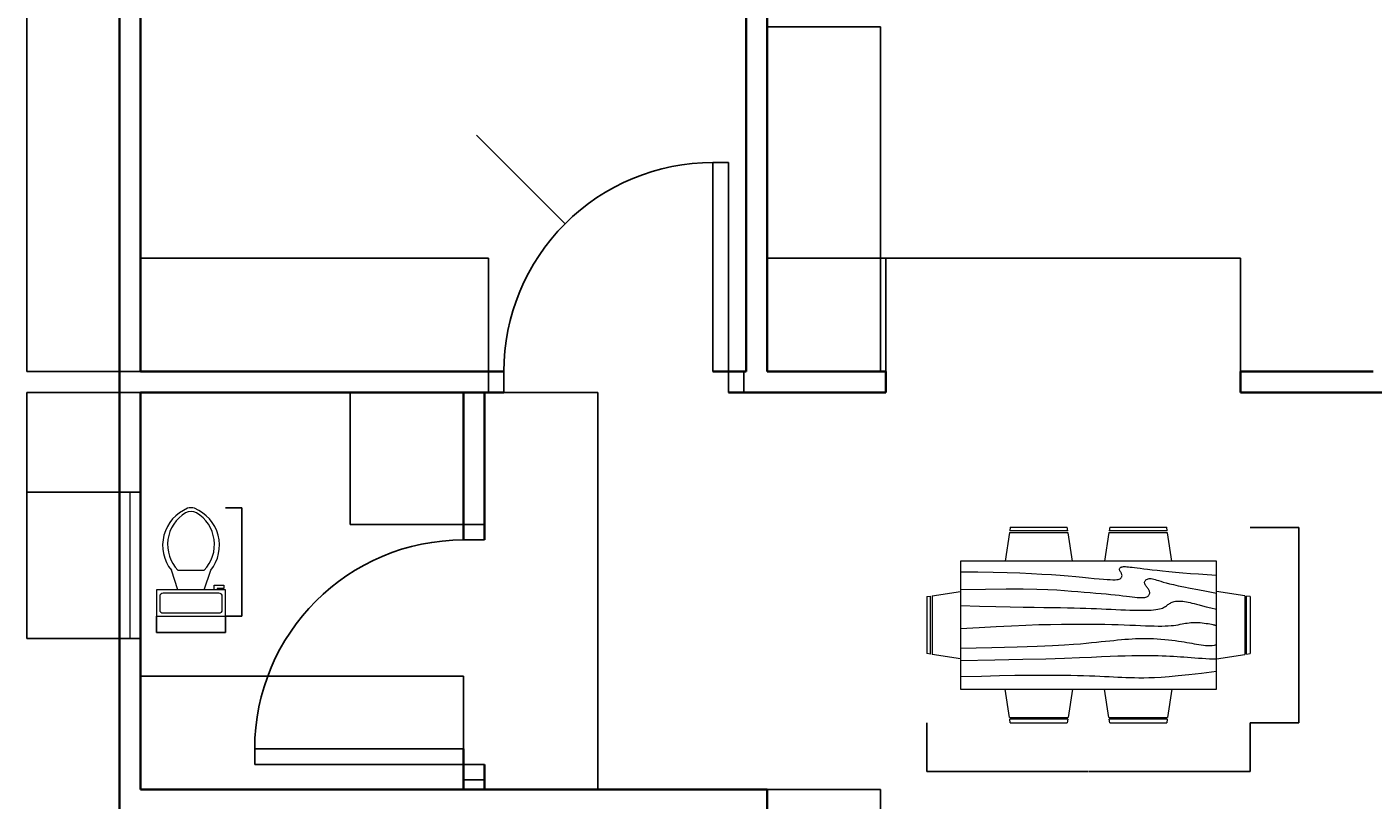
# Model space of a CAD drawing. Units: millimetres. Extents: x 1426 to 11512, y -8522 to 2664.
# Tile 2 of 4: x 1426 to 7869, y -3929 to -230. Entities that reach past the tile are written whole.
import ezdxf

# ---------------------------------------------------------------- set-up
doc = ezdxf.new("R2010")
doc.units = ezdxf.units.MM
for name, color, linetype, lineweight in [('A-ANNO-DIMS', 2, 'Continuous', 18), ('A-DOOR', 3, 'Continuous', 25), ('A-FLOR-FIXT', 9, 'Continuous', 20), ('A-FURN', 8, 'Continuous', 18), ('A-GLAZ', 4, 'Continuous', 18), ('A-WALL', 7, 'Continuous', 35)]:
    doc.layers.add(name, color=color, linetype=linetype, lineweight=lineweight)
doc.styles.get("Standard").update_dxf_attribs({"font": 'arial.ttf'})
doc.dimstyles.get("Standard").update_dxf_attribs({"dimtxt": 0.18, "dimasz": 0.18, "dimexe": 0.18, "dimexo": 0.0625, "dimgap": 0.09, "dimtad": 0, "dimtih": 1, "dimtoh": 1, "dimdec": 4, "dimzin": 0, "dimdsep": 46, "dimtxsty": 'Standard', "dimcen": 0.09, "dimadec": 0, "dimazin": 0, "dimtfac": 1, "dimtdec": 4, "dimtofl": 0, "dimtmove": 0, "dimatfit": 3, "dimfxl": 1, "dimtolj": 1, "dimtzin": 0, "dimarcsym": 0})

# ---------------------------------------------------------------- blocks, each defined once
blk = doc.blocks.new('Dining Set - 36 x 72 in.')
for p, q in [((-22, 27.5), (-22.1562, 26.50042)), ((-22, 27.5), (-6, 27.5)), ((-5.8437, 26.49966), (-6, 27.5)), ((6, 27.5), (5.8438, 26.50042)), ((6, 27.5), (22, 27.5)), ((22.1563, 26.49966), (22, 27.5)), ((-22.2343, 26.00059), (-23.4847, 17.99762)), ((-22.2304, 26), (-5.7608, 26)), ((-5.8416, 26.5), (-22.1534, 26.5)), ((-4.5152, 17.99762), (-5.7655, 25.99926)), ((5.7657, 26.00059), (4.5153, 17.99762)), ((5.7696, 26), (22.2392, 26)), ((22.1584, 26.5), (5.8466, 26.5)), ((23.4848, 17.99762), (22.2345, 25.99926)), ((36, 18), (-36, 18)), ((-36, 18), (-36, -18)), ((36, -18), (36, 18)), ((-45.5, 8), (-44.5004, 8.15617)), ((-45.5, 8), (-45.5, -8)), ((-44.5, -8.15843), (-44.5, 8.15338)), ((-44.0006, 8.23428), (-35.9976, 9.48474)), ((-44, 8.23041), (-44, -8.23915)), ((44.0006, 8.23428), (35.9976, 9.48474)), ((44, 8.23041), (44, -8.23915)), ((44.5, -8.15843), (44.5, 8.15338)), ((45.5, 8), (44.5005, 8.15617)), ((45.5, 8), (45.5, -8)), ((-44.4997, -8.15631), (-45.5, -8)), ((-35.9976, -9.48476), (-43.9993, -8.2345)), ((35.9976, -9.48476), (43.9993, -8.2345)), ((44.4997, -8.15631), (45.5, -8)), ((-36, -18), (36, -18)), ((-22.2343, -26.0006), (-23.4847, -17.99762)), ((-4.5152, -17.99762), (-5.7655, -25.99928)), ((5.7657, -26.0006), (4.5153, -17.99762)), ((23.4848, -17.99762), (22.2345, -25.99928)), ((-22.2304, -26), (-5.7608, -26)), ((-22, -27.5), (-22.1562, -26.50044)), ((-5.8416, -26.5), (-22.1534, -26.5)), ((-5.8437, -26.49967), (-6, -27.5)), ((5.7696, -26), (22.2392, -26)), ((6, -27.5), (5.8438, -26.50044)), ((22.1584, -26.5), (5.8466, -26.5)), ((22.1563, -26.49967), (22, -27.5)), ((-22, -27.5), (-6, -27.5)), ((6, -27.5), (22, -27.5))]:
    blk.add_line(p, q)
for points in [[(-36, 15), (-31.1772, 14.97754), (-26.8079, 14.91406), (-22.8538, 14.81543), (-19.276, 14.6875), (-16.0362, 14.53613), (-13.0957, 14.36718), (-10.4159, 14.18652), (-7.9583, 14), (-5.6904, 13.81315), (-3.6035, 13.63021), (-1.6954, 13.45508), (0.0365, 13.29166), (1.5945, 13.14388), (2.9811, 13.01562), (4.1988, 12.9108), (5.25, 12.83333), (6.1393, 12.78613), (6.8802, 12.76823), (7.4883, 12.77767), (7.9792, 12.8125), (8.3685, 12.87077), (8.6719, 12.95052), (8.9049, 13.0498), (9.0833, 13.16666), (9.2205, 13.29899), (9.3216, 13.44401), (9.3895, 13.59879), (9.4271, 13.76041), (9.4373, 13.92594), (9.4232, 14.09245), (9.3875, 14.257), (9.3333, 14.41666), (9.2638, 14.56917), (9.1836, 14.71484), (9.0975, 14.85465), (9.0104, 14.98958), (8.9272, 15.1206), (8.8529, 15.2487), (8.7922, 15.37483), (8.75, 15.5), (8.7305, 15.62467), (8.7344, 15.74739), (8.7617, 15.86621), (8.8125, 15.97916), (8.8867, 16.08431), (8.9844, 16.17968), (9.1055, 16.26334), (9.25, 16.33333), (9.4189, 16.38802), (9.6172, 16.42708), (9.8506, 16.45052), (10.125, 16.45833), (10.4463, 16.45052), (10.8203, 16.42708), (11.2529, 16.38802), (11.75, 16.33333), (12.3184, 16.26318), (12.9694, 16.17838), (13.7151, 16.07991), (14.5677, 15.96875), (15.5395, 15.84586), (16.6426, 15.71224), (17.8893, 15.56884), (19.2917, 15.41666), (20.859, 15.25667), (22.5879, 15.08984), (24.4721, 14.91715), (26.5052, 14.73958), (28.6809, 14.5581), (30.9929, 14.3737), (33.4347, 14.18733), (36, 14)], [(-36, 10), (-28.9766, 10.14274), (-23.1725, 10.20442), (-18.4241, 10.19775), (-14.5677, 10.13541), (-11.4399, 10.03011), (-8.877, 9.89453), (-6.7154, 9.74137), (-4.7917, 9.58333), (-2.9698, 9.43082), (-1.2246, 9.28515), (0.4415, 9.14534), (2.026, 9.01041), (3.5266, 8.87939), (4.9408, 8.7513), (6.266, 8.62516), (7.5, 8.5), (8.6411, 8.37549), (9.6914, 8.2539), (10.6538, 8.13818), (11.5312, 8.03125), (12.3267, 7.93603), (13.043, 7.85547), (13.6831, 7.79248), (14.25, 7.75), (14.7471, 7.7303), (15.1797, 7.73307), (15.5537, 7.75732), (15.875, 7.80208), (16.1494, 7.86637), (16.3828, 7.94922), (16.5811, 8.04964), (16.75, 8.16666), (16.8944, 8.29915), (17.0143, 8.44531), (17.1089, 8.60319), (17.1771, 8.77083), (17.218, 8.94629), (17.2305, 9.1276), (17.2137, 9.31282), (17.1667, 9.5), (17.0895, 9.6875), (16.987, 9.875), (16.8649, 10.0625), (16.7292, 10.25), (16.5856, 10.4375), (16.4401, 10.625), (16.2985, 10.8125), (16.1667, 11), (16.05, 11.18733), (15.9518, 11.3737), (15.8752, 11.5581), (15.8229, 11.73958), (15.798, 11.91715), (15.8034, 12.08984), (15.842, 12.25667), (15.9167, 12.41666), (16.0295, 12.56836), (16.1784, 12.70833), (16.3605, 12.83268), (16.5729, 12.9375), (16.8127, 13.01888), (17.0768, 13.07291), (17.3625, 13.0957), (17.6667, 13.08333), (17.9894, 13.03312), (18.3418, 12.94726), (18.7382, 12.82918), (19.1927, 12.68229), (19.7195, 12.51001), (20.3327, 12.31575), (21.0465, 12.10294), (21.875, 11.875), (22.8357, 11.63354), (23.959, 11.37304), (25.2786, 11.08618), (26.8282, 10.76562), (28.6414, 10.40405), (30.752, 9.99414), (33.1936, 9.52856), (36, 9)], [(-36, 5.5), (-30.7157, 5.3348), (-26.069, 5.20963), (-21.9946, 5.11767), (-18.4271, 5.05208), (-15.3009, 5.00602), (-12.5508, 4.97265), (-10.1112, 4.94515), (-7.9167, 4.91666), (-5.909, 4.88167), (-4.0586, 4.83984), (-2.3429, 4.79215), (-0.7396, 4.73958), (0.7739, 4.6831), (2.22, 4.6237), (3.6213, 4.56233), (5, 4.5), (6.373, 4.43782), (7.7344, 4.3776), (9.0723, 4.32129), (10.375, 4.27083), (11.6309, 4.22819), (12.8281, 4.19531), (13.9551, 4.17415), (15, 4.16666), (15.954, 4.17448), (16.819, 4.19791), (17.6001, 4.23698), (18.3021, 4.29166), (18.9299, 4.36198), (19.4883, 4.44791), (19.9823, 4.54948), (20.4167, 4.66666), (20.7969, 4.79899), (21.1302, 4.94401), (21.4245, 5.09879), (21.6875, 5.26041), (21.9271, 5.42594), (22.1511, 5.59245), (22.3672, 5.757), (22.5834, 5.91666), (22.8065, 6.06868), (23.0404, 6.21093), (23.2879, 6.34147), (23.5521, 6.45833), (23.8358, 6.55957), (24.142, 6.64323), (24.4735, 6.70735), (24.8334, 6.75), (25.2235, 6.76969), (25.642, 6.76692), (26.0858, 6.74267), (26.5521, 6.69791), (27.0379, 6.63362), (27.5404, 6.55078), (28.0565, 6.45036), (28.5834, 6.33333), (29.1242, 6.19987), (29.7071, 6.04687), (30.3661, 5.87044), (31.1354, 5.66666), (32.0493, 5.43164), (33.142, 5.16146), (34.4475, 4.85221), (36, 4.5)], [(-36, -1), (-30.7915, -0.6591), (-26.0195, -0.38216), (-21.6519, -0.16284), (-17.6563, 0.00521), (-14.0005, 0.12833), (-10.6523, 0.21289), (-7.5796, 0.26522), (-4.75, 0.29166), (-2.134, 0.29793), (0.2878, 0.28711), (2.5317, 0.26163), (4.6146, 0.22396), (6.5529, 0.17651), (8.3633, 0.12174), (10.0623, 0.06209), (11.6667, 0), (13.1899, -0.06201), (14.6341, -0.1211), (15.9982, -0.17432), (17.2813, -0.21875), (18.4823, -0.25147), (19.6003, -0.26953), (20.6343, -0.27002), (21.5834, -0.25), (22.4481, -0.20768), (23.2357, -0.14584), (23.9549, -0.06836), (24.6146, 0.02083), (25.2235, 0.11784), (25.7904, 0.21875), (26.3241, 0.31966), (26.8334, 0.41666), (27.3265, 0.50618), (27.8099, 0.58593), (28.2894, 0.65397), (28.7709, 0.70833), (29.2601, 0.74707), (29.763, 0.76823), (30.2855, 0.76985), (30.8334, 0.75), (31.4088, 0.70784), (31.9994, 0.64713), (32.589, 0.57275), (33.1615, 0.48958), (33.7008, 0.4025), (34.1908, 0.3164), (34.6153, 0.23616), (34.9584, 0.16666), (35.2099, 0.11165), (35.3848, 0.07031), (35.504, 0.04069), (35.5886, 0.02083), (35.6594, 0.00879), (35.7377, 0.0026), (35.8442, 0.00032), (36, 0)], [(-36, -6.5), (-27.1843, -6.31267), (-20.084, -6.1263), (-14.469, -5.9419), (-10.1094, -5.76042), (-6.7752, -5.58285), (-4.2363, -5.41016), (-2.2629, -5.24333), (-0.625, -5.08334), (0.8708, -4.93099), (2.2715, -4.78646), (3.5872, -4.64974), (4.8281, -4.52084), (6.0046, -4.39974), (7.127, -4.28646), (8.2053, -4.18099), (9.25, -4.08334), (10.2705, -3.99382), (11.2734, -3.91407), (12.2647, -3.84603), (13.25, -3.79167), (14.2354, -3.75293), (15.2266, -3.73177), (16.2295, -3.73015), (17.25, -3.75), (18.2912, -3.79248), (19.3451, -3.85547), (20.4009, -3.93604), (21.4479, -4.03125), (22.4754, -4.13819), (23.4727, -4.25391), (24.4289, -4.37549), (25.3334, -4.5), (26.1785, -4.62492), (26.9694, -4.74935), (27.7145, -4.87281), (28.4219, -4.99479), (29.1, -5.11483), (29.7572, -5.23242), (30.4016, -5.34709), (31.0417, -5.45834), (31.6837, -5.56437), (32.3262, -5.65821), (32.9658, -5.73153), (33.599, -5.77604), (34.2224, -5.78345), (34.8327, -5.74545), (35.4264, -5.65373), (36, -5.5)], [(-36, -10), (-26.4022, -9.81299), (-18.4675, -9.62891), (-11.9839, -9.45069), (-6.7396, -9.28125), (-2.5226, -9.12354), (0.8789, -8.98047), (3.6769, -8.85498), (6.0833, -8.75), (8.2767, -8.66765), (10.3021, -8.60677), (12.1712, -8.56543), (13.8958, -8.54167), (15.4876, -8.53353), (16.9583, -8.53907), (18.3197, -8.55632), (19.5834, -8.58334), (20.7616, -8.61841), (21.8685, -8.66081), (22.9188, -8.71004), (23.9271, -8.76563), (24.9081, -8.82707), (25.8763, -8.89388), (26.8465, -8.96558), (27.8334, -9.04167), (28.8474, -9.12118), (29.8828, -9.20117), (30.93, -9.27824), (31.9792, -9.34896), (33.0205, -9.40991), (34.0443, -9.45768), (35.0407, -9.48885), (36, -9.5)], [(-36, -14.5), (-30.0881, -14.33513), (-25.0332, -14.21224), (-20.7312, -14.12647), (-17.0781, -14.07292), (-13.97, -14.04671), (-11.3027, -14.04297), (-8.9724, -14.05681), (-6.875, -14.08334), (-4.9224, -14.11833), (-3.0905, -14.16016), (-1.3709, -14.20785), (0.2448, -14.26042), (1.7647, -14.3169), (3.1973, -14.3763), (4.5507, -14.43767), (5.8333, -14.5), (7.0554, -14.5621), (8.235, -14.62175), (9.3922, -14.67652), (10.5469, -14.72396), (11.7192, -14.76164), (12.929, -14.78711), (14.1965, -14.79794), (15.5417, -14.79167), (16.9933, -14.76424), (18.6152, -14.70508), (20.4804, -14.60197), (22.6615, -14.44271), (25.2312, -14.21509), (28.2624, -13.9069), (31.8277, -13.50594), (36, -13)]]:
    blk.add_lwpolyline(points)
blk = doc.blocks.new('Toilet - top')
for p, q in [((9.5, -6), (9.5, -2)), ((-8, -8.5), (-8, -8)), ((-7, -8), (-7, -9.5)), ((-4, -8), (-6, -14)), ((4, -8), (6, -14)), ((-10, -8.5), (-8, -8.5)), ((-10, -9.5), (-10, -8.5)), ((-7, -9.5), (-10, -9.5)), ((4, -14), (-4, -14))]:
    blk.add_line(p, q)
blk.add_lwpolyline([(10.5, -8), (10.5, 0), (-10.5, 0), (-10.5, -8)], close=True)
for points in [[(-9.5, -2), (-9.5, -6)], [(8.5, -1), (-8.5, -1)], [(-8.5, -7), (8.5, -7)]]:
    blk.add_lwpolyline(points)
for centre, radius, start, end in [((-8.62, -1.88), 0.884, 81.8699, 188.1301), ((8.62, -1.88), 0.884, 351.8699, 98.1301), ((-8.62, -6.12), 0.884, 171.8699, 278.1301), ((8.62, -6.12), 0.884, 261.8699, 8.1301), ((3.52, -21.58), 12.17, 141.4691, 247.9714), ((4.2, -21.82), 11.33, 136.3677, 238.9468), ((-3.52, -21.58), 12.17, 292.0284, 38.5307), ((-4.2, -21.82), 11.33, 301.053, 43.6321), ((0, -27.88), 4, 245.7318, 294.2682), ((0, -29), 4, 254.8605, 285.1395)]:
    blk.add_arc(centre, radius, start, end)
blk = doc.blocks.new('DOOR-SINGLE-1000')
for p, q in [((0, 1000), (0, 1100)), ((0, 1100), (74.2, 1100)), ((74.2, 1100), (74.2, 1000)), ((1148.4, 1000), (1148.4, 1100)), ((1148.4, 1100), (1222.6, 1100)), ((1222.6, 1100), (1222.6, 1000)), ((74.2, 1000), (0, 1000)), ((74.2, 1000), (148.4, 1000)), ((74.2, 0), (74.2, 1000)), ((148.4, 1000), (148.4, 0)), ((1222.6, 1000), (1148.4, 1000)), ((148.4, 0), (74.2, 0))]:
    blk.add_line(p, q)
blk.add_arc((148.4, 1000), 1000, 270, 0)
blk = doc.blocks.new('DOOR-LEAF-1000')
for p, q in [((1000, 74.2), (0, 74.2)), ((0, 74.2), (0, 0)), ((1000, 0), (1000, 74.2)), ((0, 0), (1000, 0))]:
    blk.add_line(p, q)
blk.add_arc((1000, 74.2), 1000, 90, 180)
blk = doc.blocks.new('*D32')
at = {"layer": 'A-ANNO-DIMS', "color": 0, "lineweight": -2, "transparency": 16777216}
for p, q in [((5733, -3559.8), (5733, -3792)), ((7280.7, -3559.8), (7280.7, -3792)), ((5733.1, -3791.8), (6505.7, -3791.8)), ((7280.5, -3791.8), (6507.9, -3791.8))]:
    blk.add_line(p, q, dxfattribs=at)
at = {"layer": 'A-ANNO-DIMS', "color": 0, "transparency": 16777216}
for points in [[(5733.1, -3791.8), (5733.1, -3791.9), (5733, -3791.8)], [(7280.5, -3791.8), (7280.5, -3791.9), (7280.7, -3791.8)]]:
    blk.add_solid(points, dxfattribs=at)
at = {"layer": 'Defpoints', "color": 0, "transparency": 16777216}
for p in [(5733, -3559.7), (7280.7, -3559.7), (7280.7, -3791.8)]:
    blk.add_point(p, dxfattribs=at)
at = {"layer": 'A-ANNO-DIMS', "color": 0, "transparency": 16777216, "insert": (6506.8, -3791.8), "char_height": 0.18, "attachment_point": 5}
blk.add_mtext('\\A1;DINING SET 1548', dxfattribs=at)
blk = doc.blocks.new('*D33')
at = {"layer": 'A-ANNO-DIMS', "color": 0, "lineweight": -2, "transparency": 16777216}
for p, q in [((7280.7, -2624.3), (7513, -2624.3)), ((7512.8, -2624.4), (7512.8, -3091.8)), ((7512.8, -3559.5), (7512.8, -3092.2)), ((7280.7, -3559.7), (7513, -3559.7))]:
    blk.add_line(p, q, dxfattribs=at)
at = {"layer": 'A-ANNO-DIMS', "color": 0, "transparency": 16777216}
for points in [[(7512.8, -2624.4), (7512.8, -2624.4), (7512.8, -2624.3)], [(7512.8, -3559.5), (7512.8, -3559.5), (7512.8, -3559.7)]]:
    blk.add_solid(points, dxfattribs=at)
at = {"layer": 'Defpoints', "color": 0, "transparency": 16777216}
for p in [(7280.7, -2624.3), (7512.8, -2624.3), (7280.7, -3559.7)]:
    blk.add_point(p, dxfattribs=at)
at = {"layer": 'A-ANNO-DIMS', "color": 0, "transparency": 16777216, "insert": (7512.8, -3092), "char_height": 0.18, "attachment_point": 5}
blk.add_mtext('\\A1;935', dxfattribs=at)
blk = doc.blocks.new('*D34')
at = {"layer": 'A-ANNO-DIMS', "color": 0, "lineweight": -2, "transparency": 16777216}
for p, q in [((2376.6, -2530.4), (2454.6, -2530.4)), ((2454.4, -2530.6), (2454.4, -2789.9)), ((2454.4, -3049.6), (2454.4, -2790.3)), ((2376.6, -3049.8), (2454.6, -3049.8))]:
    blk.add_line(p, q, dxfattribs=at)
at = {"layer": 'A-ANNO-DIMS', "color": 0, "transparency": 16777216}
for points in [[(2454.4, -2530.6), (2454.5, -2530.6), (2454.4, -2530.4)], [(2454.4, -3049.6), (2454.5, -3049.6), (2454.4, -3049.8)]]:
    blk.add_solid(points, dxfattribs=at)
at = {"layer": 'Defpoints', "color": 0, "transparency": 16777216}
for p in [(2376.5, -2530.4), (2376.5, -3049.8), (2454.4, -3049.8)]:
    blk.add_point(p, dxfattribs=at)
at = {"layer": 'A-ANNO-DIMS', "color": 0, "transparency": 16777216, "insert": (2454.4, -2790.1), "char_height": 0.18, "attachment_point": 5}
blk.add_mtext('\\A1;WC 519', dxfattribs=at)
blk = doc.blocks.new('*D35')
at = {"layer": 'A-ANNO-DIMS', "color": 0, "lineweight": -2, "transparency": 16777216}
for p, q in [((2046.5, -3049.8), (2046.5, -3127.8)), ((2376.5, -3049.8), (2376.5, -3127.8)), ((2046.7, -3127.7), (2211.3, -3127.7)), ((2376.4, -3127.7), (2211.8, -3127.7))]:
    blk.add_line(p, q, dxfattribs=at)
at = {"layer": 'A-ANNO-DIMS', "color": 0, "transparency": 16777216}
for points in [[(2046.7, -3127.6), (2046.7, -3127.7), (2046.5, -3127.7)], [(2376.4, -3127.6), (2376.4, -3127.7), (2376.5, -3127.7)]]:
    blk.add_solid(points, dxfattribs=at)
at = {"layer": 'Defpoints', "color": 0, "transparency": 16777216}
for p in [(2046.5, -3049.8), (2376.5, -3049.8), (2046.5, -3127.7)]:
    blk.add_point(p, dxfattribs=at)
at = {"layer": 'A-ANNO-DIMS', "color": 0, "transparency": 16777216, "insert": (2211.5, -3127.7), "char_height": 0.18, "attachment_point": 5}
blk.add_mtext('\\A1;330', dxfattribs=at)
blk = doc.blocks.new('*D43')
at = {"layer": 'A-ANNO-DIMS', "color": 0, "lineweight": -2, "transparency": 16777216}
for p, q in [((1968.8, 2020.9), (1426.2, 2020.9)), ((1426.4, 2020.8), (1426.4, 71.1)), ((1426.4, -1878.9), (1426.4, 70.8)), ((1968.8, -1879.1), (1426.2, -1879.1))]:
    blk.add_line(p, q, dxfattribs=at)
at = {"layer": 'A-ANNO-DIMS', "color": 0, "transparency": 16777216}
for points in [[(1426.3, 2020.8), (1426.4, 2020.8), (1426.4, 2020.9)], [(1426.3, -1878.9), (1426.4, -1878.9), (1426.4, -1879.1)]]:
    blk.add_solid(points, dxfattribs=at)
at = {"layer": 'Defpoints', "color": 0, "transparency": 16777216}
for p in [(1426.4, 2020.9), (1968.9, 2020.9), (1968.9, -1879.1)]:
    blk.add_point(p, dxfattribs=at)
at = {"layer": 'A-ANNO-DIMS', "color": 0, "transparency": 16777216, "insert": (1426.4, 70.9), "char_height": 0.18, "attachment_point": 5}
blk.add_mtext('\\A1;3900', dxfattribs=at)
blk = doc.blocks.new('*D44')
at = {"layer": 'A-ANNO-DIMS', "color": 0, "lineweight": -2, "transparency": 16777216}
for p, q in [((3616.2, -1979.1), (4158.8, -1979.1)), ((4158.6, -1979.2), (4158.6, -2928.9)), ((4158.6, -3878.9), (4158.6, -2929.2)), ((3616.2, -3879.1), (4158.8, -3879.1))]:
    blk.add_line(p, q, dxfattribs=at)
at = {"layer": 'A-ANNO-DIMS', "color": 0, "transparency": 16777216}
for points in [[(4158.6, -1979.2), (4158.7, -1979.2), (4158.6, -1979.1)], [(4158.6, -3878.9), (4158.7, -3878.9), (4158.6, -3879.1)]]:
    blk.add_solid(points, dxfattribs=at)
at = {"layer": 'Defpoints', "color": 0, "transparency": 16777216}
for p in [(3616.1, -1979.1), (3616.1, -3879.1), (4158.6, -3879.1)]:
    blk.add_point(p, dxfattribs=at)
at = {"layer": 'A-ANNO-DIMS', "color": 0, "transparency": 16777216, "insert": (4158.6, -2929.1), "char_height": 0.18, "attachment_point": 5}
blk.add_mtext('\\A1;1900', dxfattribs=at)
blk = doc.blocks.new('*D46')
at = {"layer": 'A-ANNO-DIMS', "color": 0, "lineweight": -2, "transparency": 16777216}
for p, q in [((1968.9, -3879), (1968.9, -3336.4)), ((1969.1, -3336.6), (2742, -3336.6)), ((3515.9, -3336.6), (2743, -3336.6)), ((3516.1, -3879), (3516.1, -3336.4))]:
    blk.add_line(p, q, dxfattribs=at)
at = {"layer": 'A-ANNO-DIMS', "color": 0, "transparency": 16777216}
for points in [[(1969.1, -3336.5), (1969.1, -3336.6), (1968.9, -3336.6)], [(3515.9, -3336.5), (3515.9, -3336.6), (3516.1, -3336.6)]]:
    blk.add_solid(points, dxfattribs=at)
at = {"layer": 'Defpoints', "color": 0, "transparency": 16777216}
for p in [(3516.1, -3336.6), (1968.9, -3879.1), (3516.1, -3879.1)]:
    blk.add_point(p, dxfattribs=at)
at = {"layer": 'A-ANNO-DIMS', "color": 0, "transparency": 16777216, "insert": (2742.5, -3336.6), "char_height": 0.18, "attachment_point": 5}
blk.add_mtext('\\A1;1547.3', dxfattribs=at)
blk = doc.blocks.new('*D59')
at = {"layer": 'A-ANNO-DIMS', "color": 0, "lineweight": -2, "transparency": 16777216}
for p, q in [((1968.8, -2456.2), (1426.2, -2456.2)), ((1426.4, -2456.4), (1426.4, -2806)), ((1426.4, -3156), (1426.4, -2806.4)), ((1968.8, -3156.2), (1426.2, -3156.2))]:
    blk.add_line(p, q, dxfattribs=at)
at = {"layer": 'A-ANNO-DIMS', "color": 0, "transparency": 16777216}
for points in [[(1426.3, -2456.4), (1426.4, -2456.4), (1426.4, -2456.2)], [(1426.3, -3156), (1426.4, -3156), (1426.4, -3156.2)]]:
    blk.add_solid(points, dxfattribs=at)
at = {"layer": 'Defpoints', "color": 0, "transparency": 16777216}
for p in [(1426.4, -2456.2), (1968.9, -2456.2), (1968.9, -3156.2)]:
    blk.add_point(p, dxfattribs=at)
at = {"layer": 'A-ANNO-DIMS', "color": 0, "transparency": 16777216, "insert": (1426.4, -2806.2), "char_height": 0.18, "attachment_point": 5}
blk.add_mtext('\\A1;700', dxfattribs=at)
blk = doc.blocks.new('*D60')
at = {"layer": 'A-ANNO-DIMS', "color": 0, "lineweight": -2, "transparency": 16777216}
for p, q in [((1968.8, -1979.1), (1426.2, -1979.1)), ((1426.4, -1979.2), (1426.4, -2217.4)), ((1426.4, -2456), (1426.4, -2217.8)), ((1968.8, -2456.2), (1426.2, -2456.2))]:
    blk.add_line(p, q, dxfattribs=at)
at = {"layer": 'A-ANNO-DIMS', "color": 0, "transparency": 16777216}
for points in [[(1426.3, -1979.2), (1426.4, -1979.2), (1426.4, -1979.1)], [(1426.3, -2456), (1426.4, -2456), (1426.4, -2456.2)]]:
    blk.add_solid(points, dxfattribs=at)
at = {"layer": 'Defpoints', "color": 0, "transparency": 16777216}
for p in [(1426.4, -1979.1), (1968.9, -1979.1), (1968.9, -2456.2)]:
    blk.add_point(p, dxfattribs=at)
at = {"layer": 'A-ANNO-DIMS', "color": 0, "transparency": 16777216, "insert": (1426.4, -2217.6), "char_height": 0.18, "attachment_point": 5}
blk.add_mtext('\\A1;477.1', dxfattribs=at)
blk = doc.blocks.new('*D61')
at = {"layer": 'A-ANNO-DIMS', "color": 0, "lineweight": -2, "transparency": 16777216}
for p, q in [((5537.3, -1879), (5537.3, -1336.4)), ((5537.5, -1336.6), (6385.4, -1336.6)), ((7234.3, -1336.6), (6386.3, -1336.6)), ((7234.5, -1879), (7234.5, -1336.4))]:
    blk.add_line(p, q, dxfattribs=at)
at = {"layer": 'A-ANNO-DIMS', "color": 0, "transparency": 16777216}
for points in [[(5537.5, -1336.5), (5537.5, -1336.6), (5537.3, -1336.6)], [(7234.3, -1336.5), (7234.3, -1336.6), (7234.5, -1336.6)]]:
    blk.add_solid(points, dxfattribs=at)
at = {"layer": 'Defpoints', "color": 0, "transparency": 16777216}
for p in [(7234.5, -1336.6), (5537.3, -1879.1), (7234.5, -1879.1)]:
    blk.add_point(p, dxfattribs=at)
at = {"layer": 'A-ANNO-DIMS', "color": 0, "transparency": 16777216, "insert": (6385.9, -1336.6), "char_height": 0.18, "attachment_point": 5}
blk.add_mtext('\\A1;1697.2', dxfattribs=at)
blk = doc.blocks.new('*D62')
at = {"layer": 'A-ANNO-DIMS', "color": 0, "lineweight": -2, "transparency": 16777216}
for p, q in [((4968.9, -1879), (4968.9, -1336.4)), ((4969.1, -1336.6), (5252.7, -1336.6)), ((5537.1, -1336.6), (5253.5, -1336.6)), ((5537.3, -1879), (5537.3, -1336.4))]:
    blk.add_line(p, q, dxfattribs=at)
at = {"layer": 'A-ANNO-DIMS', "color": 0, "transparency": 16777216}
for points in [[(4969.1, -1336.5), (4969.1, -1336.6), (4968.9, -1336.6)], [(5537.1, -1336.5), (5537.1, -1336.6), (5537.3, -1336.6)]]:
    blk.add_solid(points, dxfattribs=at)
at = {"layer": 'Defpoints', "color": 0, "transparency": 16777216}
for p in [(5537.3, -1336.6), (4968.9, -1879.1), (5537.3, -1879.1)]:
    blk.add_point(p, dxfattribs=at)
at = {"layer": 'A-ANNO-DIMS', "color": 0, "transparency": 16777216, "insert": (5253.1, -1336.6), "char_height": 0.18, "attachment_point": 5}
blk.add_mtext('\\A1;568.4', dxfattribs=at)
blk = doc.blocks.new('*D66')
at = {"layer": 'A-ANNO-DIMS', "color": 0, "lineweight": -2, "transparency": 16777216}
for p, q in [((4968.9, -3879.1), (5511.6, -3879.1)), ((5511.4, -3879.2), (5511.4, -4134.3)), ((5511.4, -4389.8), (5511.4, -4134.7)), ((4968.9, -4390), (5511.6, -4390))]:
    blk.add_line(p, q, dxfattribs=at)
at = {"layer": 'A-ANNO-DIMS', "color": 0, "transparency": 16777216}
for points in [[(5511.3, -3879.2), (5511.4, -3879.2), (5511.4, -3879.1)], [(5511.3, -4389.8), (5511.4, -4389.8), (5511.4, -4390)]]:
    blk.add_solid(points, dxfattribs=at)
at = {"layer": 'Defpoints', "color": 0, "transparency": 16777216}
for p in [(4968.9, -3879.1), (4968.9, -4390), (5511.4, -4390)]:
    blk.add_point(p, dxfattribs=at)
at = {"layer": 'A-ANNO-DIMS', "color": 0, "transparency": 16777216, "insert": (5511.4, -4134.5), "char_height": 0.18, "attachment_point": 5}
blk.add_mtext('\\A1;510.9', dxfattribs=at)
blk = doc.blocks.new('*D69')
at = {"layer": 'A-ANNO-DIMS', "color": 0, "lineweight": -2, "transparency": 16777216}
for p, q in [((1968.9, -1879), (1968.9, -1336.4)), ((1969.1, -1336.6), (2801.5, -1336.6)), ((3634.6, -1336.6), (2802.2, -1336.6)), ((3634.8, -1879), (3634.8, -1336.4))]:
    blk.add_line(p, q, dxfattribs=at)
at = {"layer": 'A-ANNO-DIMS', "color": 0, "transparency": 16777216}
for points in [[(1969.1, -1336.5), (1969.1, -1336.6), (1968.9, -1336.6)], [(3634.6, -1336.5), (3634.6, -1336.6), (3634.8, -1336.6)]]:
    blk.add_solid(points, dxfattribs=at)
at = {"layer": 'Defpoints', "color": 0, "transparency": 16777216}
for p in [(3634.8, -1336.6), (1968.9, -1879.1), (3634.8, -1879.1)]:
    blk.add_point(p, dxfattribs=at)
at = {"layer": 'A-ANNO-DIMS', "color": 0, "transparency": 16777216, "insert": (2801.8, -1336.6), "char_height": 0.18, "attachment_point": 5}
blk.add_mtext('\\A1;1666', dxfattribs=at)
blk = doc.blocks.new('*D72')
at = {"layer": 'A-ANNO-DIMS', "color": 0, "lineweight": -2, "transparency": 16777216}
for p, q in [((3516.1, -1979.1), (2973.4, -1979.1)), ((2973.6, -1979.2), (2973.6, -2294.5)), ((2973.6, -2610.1), (2973.6, -2294.9)), ((3516.1, -2610.3), (2973.4, -2610.3))]:
    blk.add_line(p, q, dxfattribs=at)
at = {"layer": 'A-ANNO-DIMS', "color": 0, "transparency": 16777216}
for points in [[(2973.6, -1979.2), (2973.7, -1979.2), (2973.6, -1979.1)], [(2973.6, -2610.1), (2973.7, -2610.1), (2973.6, -2610.3)]]:
    blk.add_solid(points, dxfattribs=at)
at = {"layer": 'Defpoints', "color": 0, "transparency": 16777216}
for p in [(2973.6, -1979.1), (3516.1, -1979.1), (3516.1, -2610.3)]:
    blk.add_point(p, dxfattribs=at)
at = {"layer": 'A-ANNO-DIMS', "color": 0, "transparency": 16777216, "insert": (2973.6, -2294.7), "char_height": 0.18, "attachment_point": 5}
blk.add_mtext('\\A1;631.3', dxfattribs=at)
blk = doc.blocks.new('*D73')
at = {"layer": 'A-ANNO-DIMS', "color": 0, "lineweight": -2, "transparency": 16777216}
for p, q in [((4968.9, -230.3), (5511.6, -230.3)), ((5511.4, -230.5), (5511.4, -1054.5)), ((5511.4, -1878.9), (5511.4, -1054.9)), ((4968.9, -1879.1), (5511.6, -1879.1))]:
    blk.add_line(p, q, dxfattribs=at)
at = {"layer": 'A-ANNO-DIMS', "color": 0, "transparency": 16777216}
for points in [[(5511.3, -230.5), (5511.4, -230.5), (5511.4, -230.3)], [(5511.3, -1878.9), (5511.4, -1878.9), (5511.4, -1879.1)]]:
    blk.add_solid(points, dxfattribs=at)
at = {"layer": 'Defpoints', "color": 0, "transparency": 16777216}
for p in [(4968.9, -230.3), (4968.9, -1879.1), (5511.4, -1879.1)]:
    blk.add_point(p, dxfattribs=at)
at = {"layer": 'A-ANNO-DIMS', "color": 0, "transparency": 16777216, "insert": (5511.4, -1054.7), "char_height": 0.18, "attachment_point": 5}
blk.add_mtext('\\A1;1648.8', dxfattribs=at)
blk = doc.blocks.new('*D74')
at = {"layer": 'A-ANNO-DIMS', "color": 0, "lineweight": -2, "transparency": 16777216}
for p, q in [((3577.4, -747.7), (3577.6, -747.7)), ((3577.6, -747.7), (4001.7, -1171.8)), ((4708.9, -1879.1), (4709.1, -1879.1)), ((4709, -1879.1), (4709, -1879))]:
    blk.add_line(p, q, dxfattribs=at)
at = {"layer": 'A-ANNO-DIMS', "color": 0, "transparency": 16777216}
blk.add_solid([(4001.8, -1171.8), (4001.7, -1171.8), (4001.9, -1171.9)], dxfattribs=at)
at = {"layer": 'Defpoints', "color": 0, "transparency": 16777216}
for p in [(4001.9, -1171.9), (4709, -1879.1)]:
    blk.add_point(p, dxfattribs=at)
at = {"layer": 'A-ANNO-DIMS', "color": 0, "transparency": 16777216, "insert": (3576.8, -747.7), "char_height": 0.18, "attachment_point": 5}
blk.add_mtext('\\A1;6X R1000', dxfattribs=at)

msp = doc.modelspace()

# ---------------------------------------------------------------- linework, layer by layer
at = {"layer": 'A-DOOR'}
for p, q in [((3516.12, -2610.32), (3516.12, -2684.52)), ((3616.12, -2610.32), (3516.12, -2610.32)), ((3616.12, -2684.52), (3616.12, -2610.32)), ((3616.12, -2684.52), (3616.12, -2610.32)), ((3516.12, -2684.52), (3616.12, -2684.52)), ((3516.12, -3758.72), (3516.12, -3832.92)), ((3616.12, -3758.72), (3516.12, -3758.72)), ((3516.12, -3832.92), (3616.12, -3832.92))]:
    msp.add_line(p, q, dxfattribs=at)
at = {"layer": 'A-GLAZ'}
for p, q in [((1868.87, -3156.19), (1868.87, -2456.19)), ((1868.87, -2456.19), (1968.87, -2456.19)), ((1918.87, -2456.19), (1918.87, -3156.19)), ((1968.87, -2456.19), (1968.87, -2956.19)), ((1968.87, -2956.19), (1968.87, -3056.19)), ((1968.87, -3056.19), (1968.87, -3156.19)), ((1968.87, -3156.19), (1868.87, -3156.19))]:
    msp.add_line(p, q, dxfattribs=at)
at = {"layer": 'A-WALL'}
for p, q in [((1868.87, -7979.06), (1868.87, 2120.94)), ((1968.87, -1879.06), (1968.87, 2020.94)), ((4868.87, 2020.94), (4868.87, -1879.06)), ((4968.87, 2020.94), (4968.87, -1879.06)), ((1968.87, -1879.06), (3708.98, -1879.06)), ((4708.98, -1879.06), (4868.87, -1879.06)), ((4968.87, -1879.06), (5537.29, -1879.06)), ((5537.29, -1979.06), (5537.29, -1879.06)), ((7234.46, -1879.06), (7234.46, -1979.06)), ((7234.46, -1879.06), (7868.87, -1879.06)), ((1968.87, -1979.06), (3708.98, -1979.06)), ((1968.87, -3879.06), (1968.87, -1979.06)), ((3516.12, -1979.06), (3516.12, -2684.52)), ((3616.12, -1979.06), (3616.12, -2684.52)), ((4783.18, -1979.06), (5537.29, -1979.06)), ((7234.46, -1979.06), (8081.87, -1979.06)), ((3516.12, -3684.52), (3516.12, -3879.06)), ((3616.12, -3758.72), (3616.12, -3879.06)), ((1968.87, -3879.06), (3868.87, -3879.06)), ((3868.87, -3879.06), (3968.87, -3879.06)), ((3968.87, -3879.06), (4968.87, -3879.06)), ((4968.87, -3979.06), (4968.87, -3879.06))]:
    msp.add_line(p, q, dxfattribs=at)

# ---------------------------------------------------------------- block references
at = {"layer": 'A-DOOR', "rotation": 180}
msp.add_blockref('DOOR-SINGLE-1000', (4857.38, -879.06), dxfattribs=at)
at = {"layer": 'A-DOOR'}
msp.add_blockref('DOOR-LEAF-1000', (2516.12, -3758.72), dxfattribs=at)
at = {"layer": 'A-FLOR-FIXT', "xscale": 15.71469836901466, "yscale": 15.71469836901466, "zscale": 15.71469836901466, "rotation": 180}
msp.add_blockref('Toilet - top', (2211.54, -3049.76), dxfattribs=at)
at = {"layer": 'A-FURN', "xscale": 17.00767062928736, "yscale": 17.00767062928736, "zscale": 17.00767062928736}
msp.add_blockref('Dining Set - 36 x 72 in.', (6506.81, -3091.98), dxfattribs=at)

# ---------------------------------------------------------------- dimensions: what is measured, and where the dimension line sits
at = {"layer": 'A-ANNO-DIMS'}
for base, p1, p2, angle, override, picture, middle in [((1426.37, 2020.94), (1968.87, -1879.06), (1968.87, 2020.94), 90, {"dimdec": 0, "dimlfac": 1, "dimrnd": 0, "dimzin": 0, "dimdsep": 46, "dimlunit": 2}, '*D43', (1426.37, 70.94)), ((5511.37, -1879.06), (4968.87, -230.3), (4968.87, -1879.06), 270, {"dimdec": 1, "dimlfac": 1, "dimrnd": 0, "dimzin": 0, "dimdsep": 46, "dimlunit": 2}, '*D73', (5511.37, -1054.68)), ((7234.46, -1336.56), (5537.29, -1879.06), (7234.46, -1879.06), 0, {"dimdec": 1, "dimlfac": 1, "dimrnd": 0, "dimzin": 0, "dimdsep": 46, "dimlunit": 2}, '*D61', (6385.88, -1336.56)), ((1426.37, -1979.06), (1968.87, -2456.19), (1968.87, -1979.06), 90, {"dimdec": 1, "dimlfac": 1, "dimrnd": 0, "dimzin": 0, "dimdsep": 46, "dimlunit": 2}, '*D60', (1426.37, -2217.62)), ((2973.62, -1979.06), (3516.12, -2610.32), (3516.12, -1979.06), 90, {"dimdec": 1, "dimlfac": 1, "dimrnd": 0, "dimzin": 0, "dimdsep": 46, "dimlunit": 2}, '*D72', (2973.62, -2294.69)), ((4158.62, -3879.06), (3616.12, -1979.06), (3616.12, -3879.06), 270, {"dimdec": 0, "dimlfac": 1, "dimrnd": 0, "dimzin": 0, "dimdsep": 46, "dimlunit": 2}, '*D44', (4158.62, -2929.06)), ((1426.37, -2456.19), (1968.87, -3156.19), (1968.87, -2456.19), 90, {"dimdec": 0, "dimlfac": 1, "dimrnd": 0, "dimzin": 0, "dimdsep": 46, "dimlunit": 2}, '*D59', (1426.37, -2806.19)), ((7512.82, -2624.27), (7280.66, -3559.69), (7280.66, -2624.27), 90, {"dimdec": 0, "dimlfac": 1, "dimrnd": 0, "dimzin": 0, "dimdsep": 46, "dimlunit": 2}, '*D33', (7512.82, -3091.98)), ((2046.54, -3127.66), (2376.55, -3049.76), (2046.54, -3049.76), 180, {"dimdec": 0, "dimlfac": 1, "dimrnd": 0, "dimzin": 0, "dimdsep": 46, "dimlunit": 2}, '*D35', (2211.54, -3127.66)), ((3516.1238, -3336.555), (1968.872, -3879.055), (3516.1238, -3879.055), 0, {"dimdec": 1, "dimlfac": 1, "dimrnd": 0, "dimzin": 0, "dimdsep": 46, "dimlunit": 2}, '*D46', (2742.4979, -3336.555)), ((5511.37, -4390), (4968.87, -3879.06), (4968.87, -4390), 270, {"dimdec": 1, "dimlfac": 1, "dimrnd": 0, "dimzin": 0, "dimdsep": 46, "dimlunit": 2}, '*D66', (5511.37, -4134.53))]:
    dim = msp.add_linear_dim(base=base, p1=p1, p2=p2, angle=angle, dimstyle='Standard', override=override, dxfattribs=at)
    dim.commit()
    dim.dimension.update_dxf_attribs({"geometry": picture, "text_midpoint": middle})
dim = msp.add_radius_dim(center=(4708.98, -1879.06), mpoint=(4001.87, -1171.95), text='6X <>', dimstyle='Standard', override={"dimdec": 0, "dimlfac": 1, "dimrnd": 0, "dimzin": 0, "dimdsep": 46, "dimlunit": 2}, dxfattribs=at)
dim.commit()
dim.dimension.update_dxf_attribs({"geometry": '*D74', "text_midpoint": (3576.79, -747.68), "dimtype": 164})
for base, p1, p2, override, picture, middle in [((3634.78, -1336.56), (1968.87, -1879.06), (3634.78, -1879.06), {"dimdec": 0, "dimlfac": 1, "dimrnd": 0, "dimzin": 0, "dimdsep": 46, "dimlunit": 2}, '*D69', (2801.83, -1336.56)), ((5537.29, -1336.56), (4968.87, -1879.06), (5537.29, -1879.06), {"dimdec": 1, "dimlfac": 1, "dimrnd": 0, "dimzin": 0, "dimdsep": 46, "dimlunit": 2}, '*D62', (5253.08, -1336.56))]:
    dim = msp.add_linear_dim(base=base, p1=p1, p2=p2, dimstyle='Standard', override=override, dxfattribs=at)
    dim.commit()
    dim.dimension.update_dxf_attribs({"geometry": picture, "text_midpoint": middle})
dim = msp.add_linear_dim(base=(2454.44, -3049.76), p1=(2376.55, -2530.45), p2=(2376.55, -3049.76), angle=270, text='WC <>', dimstyle='Standard', override={"dimdec": 0, "dimlfac": 1, "dimrnd": 0, "dimzin": 0, "dimdsep": 46, "dimlunit": 2}, dxfattribs=at)
dim.commit()
dim.dimension.update_dxf_attribs({"geometry": '*D34', "text_midpoint": (2454.44, -2790.11)})
dim = msp.add_linear_dim(base=(7280.66, -3791.84), p1=(5732.97, -3559.69), p2=(7280.66, -3559.69), text='DINING SET <>', dimstyle='Standard', override={"dimdec": 0, "dimlfac": 1, "dimrnd": 0, "dimzin": 0, "dimdsep": 46, "dimlunit": 2}, dxfattribs=at)
dim.commit()
dim.dimension.update_dxf_attribs({"geometry": '*D32', "text_midpoint": (6506.81, -3791.84)})

doc.saveas('drawing.dxf')
